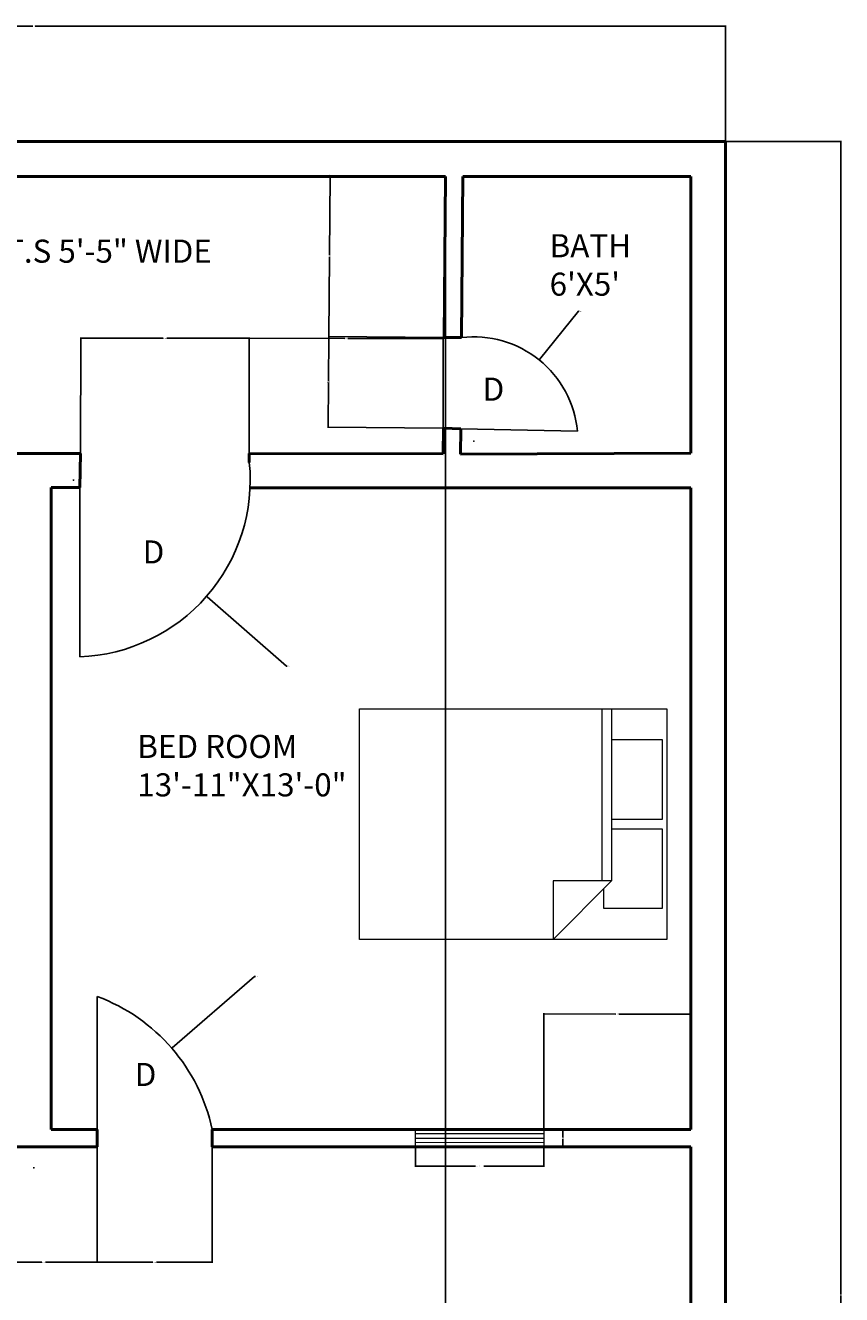
# Model space of a CAD drawing. Units: inches. Extents: x 2341 to 2761, y 2129 to 2789.
# Tile 4 of 4: x 2549 to 2761, y 2459 to 2789. Entities that reach past the tile are written whole.
import ezdxf

# ---------------------------------------------------------------- set-up
doc = ezdxf.new("R2010")
doc.units = ezdxf.units.IN
for name, color, linetype, lineweight in [('A-ANNO-DIMS', 2, 'Continuous', 18), ('A-ANNO-TEXT', 7, 'Continuous', 18), ('A-AREA-IDEN', 7, 'Continuous', 25), ('A-DOOR', 3, 'Continuous', 25), ('A-FURN', 8, 'Continuous', 18), ('A-GLAZ', 4, 'Continuous', 18), ('A-WALL', 7, 'Continuous', 50)]:
    doc.layers.add(name, color=color, linetype=linetype, lineweight=lineweight)
doc.styles.get("Standard").update_dxf_attribs({"font": 'arial.ttf'})
doc.dimstyles.get("Standard").update_dxf_attribs({"dimtxt": 0.18, "dimasz": 0.18, "dimexe": 0.18, "dimexo": 0.0625, "dimgap": 0.09, "dimtad": 0, "dimtih": 1, "dimtoh": 1, "dimdec": 4, "dimzin": 0, "dimdsep": 46, "dimtxsty": 'Standard', "dimcen": 0.09, "dimadec": 0, "dimazin": 0, "dimtfac": 1, "dimtdec": 4, "dimtofl": 0, "dimtmove": 0, "dimatfit": 3, "dimfxl": 1, "dimtolj": 1, "dimtzin": 0, "dimarcsym": 0})

# ---------------------------------------------------------------- blocks, each defined once
blk = doc.blocks.new('Bed - Queen')
for p, q in [((0, -80.00003), (0, 0)), ((0, 0), (59.99999, 0)), ((59.99999, 0), (59.99999, -80.00003)), ((7.99999, -1.2), (28.79998, -1.2)), ((7.99999, -14.4), (7.99999, -1.2)), ((28.79998, -1.2), (28.79998, -14.4)), ((31.19999, -1.2), (51.99999, -1.2)), ((31.19999, -14.4), (31.19999, -1.2)), ((51.99999, -1.2), (51.99999, -16.4)), ((0, -14.4), (44.8, -14.4)), ((59.99999, -29.6), (44.8, -14.4)), ((44.8, -14.4), (44.8, -29.6)), ((51.99999, -16.4), (46.79936, -16.4)), ((44.8, -16.8), (0, -16.8)), ((44.8, -29.6), (59.99999, -29.6)), ((59.99999, -80.00003), (0, -80.00003))]:
    blk.add_line(p, q)
blk = doc.blocks.new('WIN-33IN-NARROW')
for p, q in [((0, 3.43), (33.34, 3.43)), ((0, 2.27), (33.34, 2.27)), ((0, 1.23), (33.34, 1.12))]:
    blk.add_line(p, q)
blk.add_lwpolyline([(0, 4.54), (33.34, 4.54), (33.34, 0), (0, 0)], close=True)
blk = doc.blocks.new('*D5')
at = {"layer": 'A-ANNO-DIMS', "color": 0, "lineweight": -2, "transparency": 16777216}
for p, q in [((2650.57, 2497.53), (2650.57, 2492.41)), ((2683.92, 2497.53), (2683.92, 2492.41)), ((2650.75, 2492.59), (2666.13, 2492.59)), ((2683.74, 2492.59), (2668.37, 2492.59))]:
    blk.add_line(p, q, dxfattribs=at)
at = {"layer": 'A-ANNO-DIMS', "color": 0, "transparency": 16777216}
for points in [[(2650.75, 2492.62), (2650.75, 2492.56), (2650.57, 2492.59)], [(2683.74, 2492.62), (2683.74, 2492.56), (2683.92, 2492.59)]]:
    blk.add_solid(points, dxfattribs=at)
at = {"layer": 'Defpoints', "color": 0, "transparency": 16777216}
for p in [(2650.57, 2497.6), (2683.92, 2497.6), (2683.92, 2492.59)]:
    blk.add_point(p, dxfattribs=at)
at = {"layer": 'A-ANNO-DIMS', "color": 0, "transparency": 16777216, "insert": (2667.25, 2492.59), "char_height": 0.18, "attachment_point": 5}
blk.add_mtext('\\A1;WINDOW 33 TYP.', dxfattribs=at)
blk = doc.blocks.new('*D6')
at = {"layer": 'A-ANNO-DIMS', "color": 0, "lineweight": -2, "transparency": 16777216}
for p, q in [((2683.98, 2502.14), (2689.1, 2502.14)), ((2688.92, 2501.96), (2688.92, 2500.05)), ((2683.98, 2497.6), (2689.1, 2497.6)), ((2688.92, 2497.78), (2688.92, 2499.68))]:
    blk.add_line(p, q, dxfattribs=at)
at = {"layer": 'A-ANNO-DIMS', "color": 0, "transparency": 16777216}
for points in [[(2688.89, 2501.96), (2688.95, 2501.96), (2688.92, 2502.14)], [(2688.89, 2497.78), (2688.95, 2497.78), (2688.92, 2497.6)]]:
    blk.add_solid(points, dxfattribs=at)
at = {"layer": 'Defpoints', "color": 0, "transparency": 16777216}
for p in [(2683.92, 2502.14), (2688.92, 2502.14), (2683.92, 2497.6)]:
    blk.add_point(p, dxfattribs=at)
at = {"layer": 'A-ANNO-DIMS', "color": 0, "transparency": 16777216, "insert": (2688.92, 2499.87), "char_height": 0.18, "attachment_point": 5}
blk.add_mtext('\\A1;5 TYP.', dxfattribs=at)
blk = doc.blocks.new('*D11')
at = {"layer": 'A-ANNO-DIMS', "color": 0, "lineweight": -2, "transparency": 16777216}
for p, q in [((2371.24, 2759.18), (2371.24, 2789.36)), ((2371.42, 2789.18), (2550.95, 2789.18)), ((2731.06, 2789.18), (2551.53, 2789.18)), ((2731.24, 2759.18), (2731.24, 2789.36))]:
    blk.add_line(p, q, dxfattribs=at)
at = {"layer": 'A-ANNO-DIMS', "color": 0, "transparency": 16777216}
for points in [[(2371.42, 2789.21), (2371.42, 2789.15), (2371.24, 2789.18)], [(2731.06, 2789.21), (2731.06, 2789.15), (2731.24, 2789.18)]]:
    blk.add_solid(points, dxfattribs=at)
at = {"layer": 'Defpoints', "color": 0, "transparency": 16777216}
for p in [(2731.24, 2789.18), (2371.24, 2759.12), (2731.24, 2759.12)]:
    blk.add_point(p, dxfattribs=at)
at = {"layer": 'A-ANNO-DIMS', "color": 0, "transparency": 16777216, "insert": (2551.24, 2789.18), "char_height": 0.18, "attachment_point": 5}
blk.add_mtext('\\A1;360', dxfattribs=at)
blk = doc.blocks.new('*D12')
at = {"layer": 'A-ANNO-DIMS', "color": 0, "lineweight": -2, "transparency": 16777216}
for p, q in [((2731.3, 2759.12), (2761.44, 2759.12)), ((2761.26, 2758.94), (2761.26, 2459.3)), ((2761.26, 2159.3), (2761.26, 2458.94)), ((2731.3, 2159.12), (2761.44, 2159.12))]:
    blk.add_line(p, q, dxfattribs=at)
at = {"layer": 'A-ANNO-DIMS', "color": 0, "transparency": 16777216}
for points in [[(2761.23, 2758.94), (2761.29, 2758.94), (2761.26, 2759.12)], [(2761.23, 2159.3), (2761.29, 2159.3), (2761.26, 2159.12)]]:
    blk.add_solid(points, dxfattribs=at)
at = {"layer": 'Defpoints', "color": 0, "transparency": 16777216}
for p in [(2731.24, 2759.12), (2761.26, 2759.12), (2731.24, 2159.12)]:
    blk.add_point(p, dxfattribs=at)
at = {"layer": 'A-ANNO-DIMS', "color": 0, "transparency": 16777216, "insert": (2761.26, 2459.12), "char_height": 0.18, "attachment_point": 5}
blk.add_mtext('\\A1;600', dxfattribs=at)
blk = doc.blocks.new('*D17')
at = {"layer": 'A-ANNO-DIMS', "color": 0, "lineweight": -2, "transparency": 16777216}
for p, q in [((2444.74, 2750.05), (2444.74, 2128.92)), ((2658.39, 2749.97), (2658.39, 2128.92)), ((2444.92, 2129.1), (2551.1, 2129.1)), ((2658.21, 2129.1), (2552.03, 2129.1))]:
    blk.add_line(p, q, dxfattribs=at)
at = {"layer": 'A-ANNO-DIMS', "color": 0, "transparency": 16777216}
for points in [[(2444.92, 2129.13), (2444.92, 2129.07), (2444.74, 2129.1)], [(2658.21, 2129.13), (2658.21, 2129.07), (2658.39, 2129.1)]]:
    blk.add_solid(points, dxfattribs=at)
at = {"layer": 'Defpoints', "color": 0, "transparency": 16777216}
for p in [(2444.74, 2750.12), (2658.39, 2750.04), (2658.39, 2129.1)]:
    blk.add_point(p, dxfattribs=at)
at = {"layer": 'A-ANNO-DIMS', "color": 0, "transparency": 16777216, "insert": (2551.56, 2129.1), "char_height": 0.18, "attachment_point": 5}
blk.add_mtext('\\A1;213.65', dxfattribs=at)
blk = doc.blocks.new('*D34')
at = {"layer": 'A-ANNO-DIMS', "color": 0, "lineweight": -2, "transparency": 16777216}
for p, q in [((2683.92, 2502.2), (2683.95, 2532.34)), ((2684.13, 2532.16), (2702.72, 2532.14)), ((2722.09, 2532.12), (2703.51, 2532.14)), ((2722.24, 2502.16), (2722.27, 2532.3))]:
    blk.add_line(p, q, dxfattribs=at)
at = {"layer": 'A-ANNO-DIMS', "color": 0, "transparency": 16777216}
for points in [[(2684.13, 2532.19), (2684.13, 2532.13), (2683.95, 2532.16)], [(2722.09, 2532.15), (2722.09, 2532.09), (2722.27, 2532.12)]]:
    blk.add_solid(points, dxfattribs=at)
at = {"layer": 'Defpoints', "color": 0, "transparency": 16777216}
for p in [(2722.27, 2532.12), (2683.92, 2502.14), (2722.24, 2502.1)]:
    blk.add_point(p, dxfattribs=at)
at = {"layer": 'A-ANNO-DIMS', "color": 0, "transparency": 16777216, "insert": (2703.11, 2532.14), "char_height": 0.18, "attachment_point": 5}
blk.add_mtext('\\A1;38.32', dxfattribs=at)
blk = doc.blocks.new('*D39')
at = {"layer": 'A-ANNO-DIMS', "color": 0, "lineweight": -2, "transparency": 16777216}
for p, q in [((2628.37, 2750.12), (2628.18, 2729.54)), ((2658.32, 2750.04), (2628.19, 2750.31)), ((2628, 2708.6), (2628.18, 2729.18)), ((2657.95, 2708.15), (2627.81, 2708.42))]:
    blk.add_line(p, q, dxfattribs=at)
at = {"layer": 'A-ANNO-DIMS', "color": 0, "transparency": 16777216}
for points in [[(2628.34, 2750.13), (2628.4, 2750.12), (2628.37, 2750.3)], [(2627.97, 2708.6), (2628.03, 2708.6), (2627.99, 2708.42)]]:
    blk.add_solid(points, dxfattribs=at)
at = {"layer": 'Defpoints', "color": 0, "transparency": 16777216}
for p in [(2628.37, 2750.3), (2658.39, 2750.04), (2658.01, 2708.15)]:
    blk.add_point(p, dxfattribs=at)
at = {"layer": 'A-ANNO-DIMS', "color": 0, "transparency": 16777216, "insert": (2628.18, 2729.36), "char_height": 0.18, "attachment_point": 5}
blk.add_mtext('\\A1;41.89', dxfattribs=at)
blk = doc.blocks.new('*D40')
at = {"layer": 'A-ANNO-DIMS', "color": 0, "lineweight": -2, "transparency": 16777216}
for p, q in [((2657.95, 2708.15), (2627.81, 2708.42)), ((2627.99, 2708.24), (2627.89, 2696.79)), ((2627.78, 2684.98), (2627.89, 2696.43)), ((2657.74, 2684.53), (2627.6, 2684.8))]:
    blk.add_line(p, q, dxfattribs=at)
at = {"layer": 'A-ANNO-DIMS', "color": 0, "transparency": 16777216}
for points in [[(2627.96, 2708.24), (2628.02, 2708.24), (2627.99, 2708.42)], [(2627.75, 2684.98), (2627.81, 2684.98), (2627.78, 2684.8)]]:
    blk.add_solid(points, dxfattribs=at)
at = {"layer": 'Defpoints', "color": 0, "transparency": 16777216}
for p in [(2627.99, 2708.42), (2658.01, 2708.15), (2657.8, 2684.53)]:
    blk.add_point(p, dxfattribs=at)
at = {"layer": 'A-ANNO-DIMS', "color": 0, "transparency": 16777216, "insert": (2627.89, 2696.61), "char_height": 0.18, "attachment_point": 5}
blk.add_mtext('\\A1;23.616', dxfattribs=at)
blk = doc.blocks.new('*D41')
at = {"layer": 'A-ANNO-DIMS', "color": 0, "lineweight": -2, "transparency": 16777216}
for p, q in [((2563.36, 2678.05), (2563.4, 2708.19)), ((2563.58, 2708.01), (2584.86, 2707.98)), ((2607.07, 2707.96), (2585.79, 2707.98)), ((2607.22, 2678), (2607.25, 2708.14))]:
    blk.add_line(p, q, dxfattribs=at)
at = {"layer": 'A-ANNO-DIMS', "color": 0, "transparency": 16777216}
for points in [[(2563.58, 2708.04), (2563.58, 2707.98), (2563.4, 2708.01)], [(2607.07, 2707.99), (2607.07, 2707.93), (2607.25, 2707.96)]]:
    blk.add_solid(points, dxfattribs=at)
at = {"layer": 'Defpoints', "color": 0, "transparency": 16777216}
for p in [(2607.25, 2707.96), (2563.36, 2677.99), (2607.22, 2677.94)]:
    blk.add_point(p, dxfattribs=at)
at = {"layer": 'A-ANNO-DIMS', "color": 0, "transparency": 16777216, "insert": (2585.32, 2707.98), "char_height": 0.18, "attachment_point": 5}
blk.add_mtext('\\A1;43.855', dxfattribs=at)
blk = doc.blocks.new('*D42')
at = {"layer": 'A-ANNO-DIMS', "color": 0, "lineweight": -2, "transparency": 16777216}
for p, q in [((2607.22, 2678), (2607.25, 2708.14)), ((2607.43, 2707.96), (2632.12, 2707.93)), ((2657.6, 2707.9), (2632.91, 2707.93)), ((2657.74, 2677.94), (2657.78, 2708.08))]:
    blk.add_line(p, q, dxfattribs=at)
at = {"layer": 'A-ANNO-DIMS', "color": 0, "transparency": 16777216}
for points in [[(2607.43, 2707.99), (2607.43, 2707.93), (2607.25, 2707.96)], [(2657.6, 2707.93), (2657.6, 2707.87), (2657.78, 2707.9)]]:
    blk.add_solid(points, dxfattribs=at)
at = {"layer": 'Defpoints', "color": 0, "transparency": 16777216}
for p in [(2657.78, 2707.9), (2607.22, 2677.94), (2657.74, 2677.88)]:
    blk.add_point(p, dxfattribs=at)
at = {"layer": 'A-ANNO-DIMS', "color": 0, "transparency": 16777216, "insert": (2632.51, 2707.93), "char_height": 0.18, "attachment_point": 5}
blk.add_mtext('\\A1;50.52', dxfattribs=at)
blk = doc.blocks.new('*D45')
at = {"layer": 'A-ANNO-DIMS', "color": 0, "lineweight": -2, "transparency": 16777216}
for p, q in [((2539.74, 2497.53), (2539.74, 2467.4)), ((2567.7, 2497.53), (2567.7, 2467.4)), ((2539.92, 2467.58), (2553.25, 2467.58)), ((2567.52, 2467.58), (2554.19, 2467.58))]:
    blk.add_line(p, q, dxfattribs=at)
at = {"layer": 'A-ANNO-DIMS', "color": 0, "transparency": 16777216}
for points in [[(2539.92, 2467.61), (2539.92, 2467.55), (2539.74, 2467.58)], [(2567.52, 2467.61), (2567.52, 2467.55), (2567.7, 2467.58)]]:
    blk.add_solid(points, dxfattribs=at)
at = {"layer": 'Defpoints', "color": 0, "transparency": 16777216}
for p in [(2539.74, 2497.6), (2567.7, 2497.6), (2539.74, 2467.58)]:
    blk.add_point(p, dxfattribs=at)
at = {"layer": 'A-ANNO-DIMS', "color": 0, "transparency": 16777216, "insert": (2553.72, 2467.58), "char_height": 0.18, "attachment_point": 5}
blk.add_mtext('\\A1;27.967', dxfattribs=at)
blk = doc.blocks.new('*D46')
at = {"layer": 'A-ANNO-DIMS', "color": 0, "lineweight": -2, "transparency": 16777216}
for p, q in [((2567.7, 2497.53), (2567.7, 2467.4)), ((2597.63, 2497.53), (2597.63, 2467.4)), ((2567.88, 2467.58), (2582.2, 2467.58)), ((2597.45, 2467.58), (2583.13, 2467.58))]:
    blk.add_line(p, q, dxfattribs=at)
at = {"layer": 'A-ANNO-DIMS', "color": 0, "transparency": 16777216}
for points in [[(2567.88, 2467.61), (2567.88, 2467.55), (2567.7, 2467.58)], [(2597.45, 2467.61), (2597.45, 2467.55), (2597.63, 2467.58)]]:
    blk.add_solid(points, dxfattribs=at)
at = {"layer": 'Defpoints', "color": 0, "transparency": 16777216}
for p in [(2567.7, 2497.6), (2597.63, 2497.6), (2567.7, 2467.58)]:
    blk.add_point(p, dxfattribs=at)
at = {"layer": 'A-ANNO-DIMS', "color": 0, "transparency": 16777216, "insert": (2582.67, 2467.58), "char_height": 0.18, "attachment_point": 5}
blk.add_mtext('\\A1;29.925', dxfattribs=at)
blk = doc.blocks.new('*D65')
at = {"layer": 'A-ANNO-DIMS', "color": 0, "lineweight": -2, "transparency": 16777216}
for p, q in [((2608.67, 2541.89), (2587.24, 2523.36)), ((2608.85, 2541.89), (2608.67, 2541.89)), ((2551.08, 2492.17), (2551.26, 2492.17)), ((2551.17, 2492.08), (2551.17, 2492.26))]:
    blk.add_line(p, q, dxfattribs=at)
at = {"layer": 'A-ANNO-DIMS', "color": 0, "transparency": 16777216}
blk.add_solid([(2587.22, 2523.38), (2587.26, 2523.34), (2587.11, 2523.24)], dxfattribs=at)
at = {"layer": 'Defpoints', "color": 0, "transparency": 16777216}
for p in [(2587.11, 2523.24), (2551.17, 2492.17)]:
    blk.add_point(p, dxfattribs=at)
at = {"layer": 'A-ANNO-DIMS', "color": 0, "transparency": 16777216, "insert": (2609.31, 2541.89), "char_height": 0.18, "attachment_point": 5}
blk.add_mtext('\\A1;R47.51', dxfattribs=at)
blk = doc.blocks.new('*D66')
at = {"layer": 'A-ANNO-DIMS', "color": 0, "lineweight": -2, "transparency": 16777216}
for p, q in [((2561.4, 2671.08), (2561.58, 2671.08)), ((2561.49, 2670.99), (2561.49, 2671.17)), ((2616.98, 2622.68), (2596.31, 2640.71)), ((2617.16, 2622.68), (2616.98, 2622.68))]:
    blk.add_line(p, q, dxfattribs=at)
at = {"layer": 'A-ANNO-DIMS', "color": 0, "transparency": 16777216}
blk.add_solid([(2596.33, 2640.74), (2596.29, 2640.69), (2596.18, 2640.83)], dxfattribs=at)
at = {"layer": 'Defpoints', "color": 0, "transparency": 16777216}
for p in [(2561.49, 2671.08), (2596.18, 2640.83)]:
    blk.add_point(p, dxfattribs=at)
at = {"layer": 'A-ANNO-DIMS', "color": 0, "transparency": 16777216, "insert": (2617.64, 2622.68), "char_height": 0.18, "attachment_point": 5}
blk.add_mtext('\\A1;R46.02', dxfattribs=at)
blk = doc.blocks.new('*D71')
at = {"layer": 'A-ANNO-DIMS', "color": 0, "lineweight": -2, "transparency": 16777216}
for p, q in [((2692.96, 2715), (2682.84, 2702.47)), ((2693.14, 2715), (2692.96, 2715)), ((2665.6, 2681.2), (2665.78, 2681.2)), ((2665.69, 2681.11), (2665.69, 2681.29))]:
    blk.add_line(p, q, dxfattribs=at)
at = {"layer": 'A-ANNO-DIMS', "color": 0, "transparency": 16777216}
blk.add_solid([(2682.82, 2702.48), (2682.87, 2702.45), (2682.73, 2702.33)], dxfattribs=at)
at = {"layer": 'Defpoints', "color": 0, "transparency": 16777216}
for p in [(2682.73, 2702.33), (2665.69, 2681.2)]:
    blk.add_point(p, dxfattribs=at)
at = {"layer": 'A-ANNO-DIMS', "color": 0, "transparency": 16777216, "insert": (2693.62, 2715), "char_height": 0.18, "attachment_point": 5}
blk.add_mtext('\\A1;R27.14', dxfattribs=at)

msp = doc.modelspace()

# ---------------------------------------------------------------- linework, layer by layer
at = {"layer": 'A-DOOR'}
for p, q in [((2662.3014, 2684.4386), (2692.7079, 2683.7981)), ((2563.168, 2669.0935), (2563.168, 2625.0916)), ((2567.7033, 2502.0958), (2567.7033, 2536.7085))]:
    msp.add_line(p, q, dxfattribs=at)
for centre, radius, start, end in [((2665.69, 2681.2001), 27.1425, 5.492613, 96.721177), ((2561.4946, 2671.0796), 46.0184, 272.083846, 5.728137), ((2551.1668, 2492.1696), 47.5097, 12.059661, 69.630976)]:
    msp.add_arc(centre, radius, start, end, dxfattribs=at)
at = {"layer": 'A-WALL'}
for p, q in [((2371.242, 2759.1219), (2731.242, 2759.1219)), ((2658.4684, 2759.1219), (2658.4688, 2759.1621)), ((2731.242, 2759.1219), (2731.242, 2159.1219)), ((2444.742, 2750.1173), (2658.3873, 2750.0366)), ((2658.013, 2708.1489), (2658.3873, 2750.0366)), ((2662.5133, 2708.1561), (2662.8874, 2750.0349)), ((2662.8874, 2750.0349), (2722.242, 2750.0125)), ((2722.242, 2750.0125), (2722.242, 2678.0627)), ((2658.013, 2708.1489), (2662.5133, 2708.1561)), ((2657.7426, 2677.8811), (2657.8021, 2684.5334)), ((2657.8021, 2684.5334), (2662.3014, 2684.4386)), ((2662.2425, 2677.8409), (2662.3014, 2684.4386)), ((2444.742, 2678.1173), (2563.3637, 2677.9857)), ((2563.3637, 2677.9857), (2563.168, 2669.0935)), ((2607.2192, 2677.9371), (2607.2833, 2675.6727)), ((2607.2192, 2677.9371), (2657.7426, 2677.8811)), ((2722.242, 2678.0627), (2662.2425, 2677.8409)), ((2555.742, 2669.0958), (2555.742, 2502.0958)), ((2555.742, 2669.0958), (2555.742, 2502.0958)), ((2555.742, 2669.0949), (2563.168, 2669.0935)), ((2607.4698, 2669.0849), (2722.242, 2669.0627)), ((2722.242, 2669.0627), (2722.242, 2502.0958)), ((2555.742, 2502.0958), (2567.7033, 2502.0958)), ((2567.7033, 2502.0958), (2567.7033, 2497.5958)), ((2597.628, 2502.0958), (2597.628, 2497.5958)), ((2597.628, 2502.0958), (2722.242, 2502.0958)), ((2551.242, 2497.5958), (2539.7368, 2497.5958)), ((2551.242, 2497.5958), (2567.7033, 2497.5958)), ((2597.628, 2497.5958), (2722.242, 2497.5958)), ((2722.2419, 2497.5958), (2722.2379, 2346.0958))]:
    msp.add_line(p, q, dxfattribs=at)

# ---------------------------------------------------------------- block references
at = {"layer": 'A-FURN', "rotation": 270}
msp.add_blockref('Bed - Queen', (2715.9364, 2611.5597), dxfattribs=at)
at = {"layer": 'A-GLAZ'}
msp.add_blockref('WIN-33IN-NARROW', (2650.5749, 2497.5959), dxfattribs=at)

# ---------------------------------------------------------------- texts
at = {"layer": 'A-ANNO-TEXT', "char_height": 6, "attachment_point": 1}
for insert in [(2668.0113, 2697.7097), (2579.5205, 2655.3659), (2577.4571, 2519.4181)]:
    msp.add_mtext_dynamic_manual_height_columns('D', width=9.002909, gutter_width=12.5, heights=[0], dxfattribs=dict(at, insert=insert))
at = {"layer": 'A-AREA-IDEN', "char_height": 6, "attachment_point": 1}
for s, width, insert in [("BATH\\P6'X5'", 24.899212, (2685.4527, 2735.0332)), ('O.T.S 5\'-5" WIDE ', 77.771128, (2535.3365, 2733.6222)), ('BED ROOM \\P13\'-11"X13\'-0"', 65.352086, (2578.1157, 2604.7685))]:
    msp.add_mtext_dynamic_manual_height_columns(s, width=width, gutter_width=12.5, heights=[0], dxfattribs=dict(at, insert=insert))

# ---------------------------------------------------------------- dimensions: what is measured, and where the dimension line sits
at = {"layer": 'A-ANNO-DIMS'}
for base, p1, p2, override, picture, middle in [((2731.242, 2789.1821), (2371.242, 2759.1219), (2731.242, 2759.1219), {"dimdec": 0, "dimlfac": 1, "dimrnd": 0, "dimzin": 0, "dimdsep": 46, "dimlunit": 2}, '*D11', (2551.242, 2789.1821)), ((2658.3873, 2129.1019), (2444.742, 2750.1173), (2658.3873, 2750.0366), {"dimdec": 2, "dimlfac": 1, "dimrnd": 0, "dimzin": 0, "dimdsep": 46, "dimlunit": 2}, '*D17', (2551.5646, 2129.1019))]:
    dim = msp.add_linear_dim(base=base, p1=p1, p2=p2, dimstyle='Standard', override=override, dxfattribs=at)
    dim.commit()
    dim.dimension.update_dxf_attribs({"geometry": picture, "text_midpoint": middle})
for base, p1, p2, angle, override, picture, middle in [((2761.262, 2759.1219), (2731.242, 2159.1219), (2731.242, 2759.1219), 90, {"dimdec": 0, "dimlfac": 1, "dimrnd": 0, "dimzin": 0, "dimdsep": 46, "dimlunit": 2}, '*D12', (2761.262, 2459.1219)), ((2628.3685, 2750.3048), (2658.013, 2708.1489), (2658.3873, 2750.0366), 89.488145, {"dimdec": 2, "dimlfac": 1, "dimrnd": 0, "dimzin": 0, "dimdsep": 46, "dimlunit": 2}, '*D39', (2628.1813, 2729.3609)), ((2607.25246, 2707.95707), (2563.36371, 2677.98573), (2607.21916, 2677.93709), 359.936454, {"dimdec": 3, "dimlfac": 1, "dimrnd": 0, "dimzin": 0, "dimdsep": 46, "dimlunit": 2}, '*D41', (2585.32473, 2707.98139)), ((2657.7759, 2707.901), (2607.2192, 2677.9371), (2657.7426, 2677.8811), 359.936454, {"dimdec": 2, "dimlfac": 1, "dimrnd": 0, "dimzin": 0, "dimdsep": 46, "dimlunit": 2}, '*D42', (2632.5142, 2707.9291)), ((2627.9942, 2708.4171), (2657.8021, 2684.5334), (2658.013, 2708.1489), 89.488145, {"dimdec": 3, "dimlfac": 1, "dimrnd": 0, "dimzin": 0, "dimdsep": 46, "dimlunit": 2}, '*D40', (2627.8887, 2696.6093)), ((2722.2743, 2532.1158), (2683.9199, 2502.1369), (2722.242, 2502.0958), 359.938506, {"dimdec": 2, "dimlfac": 1, "dimrnd": 0, "dimzin": 0, "dimdsep": 46, "dimlunit": 2}, '*D34', (2703.1132, 2532.1363)), ((2539.73676, 2467.57579), (2567.70327, 2497.59579), (2539.73676, 2497.59579), 180, {"dimdec": 3, "dimlfac": 1, "dimrnd": 0, "dimzin": 0, "dimdsep": 46, "dimlunit": 2}, '*D45', (2553.72001, 2467.57579)), ((2567.7033, 2467.5758), (2597.628, 2497.5958), (2567.7033, 2497.5958), 180, {"dimdec": 3, "dimlfac": 1, "dimrnd": 0, "dimzin": 0, "dimdsep": 46, "dimlunit": 2}, '*D46', (2582.6656, 2467.5758))]:
    dim = msp.add_linear_dim(base=base, p1=p1, p2=p2, angle=angle, dimstyle='Standard', override=override, dxfattribs=at)
    dim.commit()
    dim.dimension.update_dxf_attribs({"geometry": picture, "text_midpoint": middle})
for center, mpoint, picture, middle in [((2665.69, 2681.2001), (2682.7318, 2702.3257), '*D71', (2693.6163, 2715.0011)), ((2561.4946, 2671.0796), (2596.1758, 2640.8321), '*D66', (2617.6435, 2622.6837)), ((2551.1668, 2492.1696), (2587.1068, 2523.2418), '*D65', (2609.3133, 2541.8852))]:
    dim = msp.add_radius_dim(center=center, mpoint=mpoint, dimstyle='Standard', override={"dimdec": 2, "dimlfac": 1, "dimrnd": 0, "dimzin": 0, "dimdsep": 46, "dimlunit": 2}, dxfattribs=at)
    dim.commit()
    dim.dimension.update_dxf_attribs({"geometry": picture, "text_midpoint": middle, "dimtype": 164})
dim = msp.add_linear_dim(base=(2688.9217, 2502.1369), p1=(2683.9199, 2497.5958), p2=(2683.9199, 2502.1369), angle=90, text='<> TYP.', dimstyle='Standard', override={"dimdec": 0, "dimlfac": 1, "dimrnd": 0, "dimzin": 0, "dimdsep": 46, "dimlunit": 2}, dxfattribs=at)
dim.commit()
dim.dimension.update_dxf_attribs({"geometry": '*D6', "text_midpoint": (2688.9217, 2499.8664)})
dim = msp.add_linear_dim(base=(2683.9199, 2492.594), p1=(2650.5745, 2497.5958), p2=(2683.9199, 2497.5958), text='WINDOW <> TYP.', dimstyle='Standard', override={"dimdec": 0, "dimlfac": 1, "dimrnd": 0, "dimzin": 0, "dimdsep": 46, "dimlunit": 2}, dxfattribs=at)
dim.commit()
dim.dimension.update_dxf_attribs({"geometry": '*D5', "text_midpoint": (2667.2472, 2492.594)})

doc.saveas('drawing.dxf')
